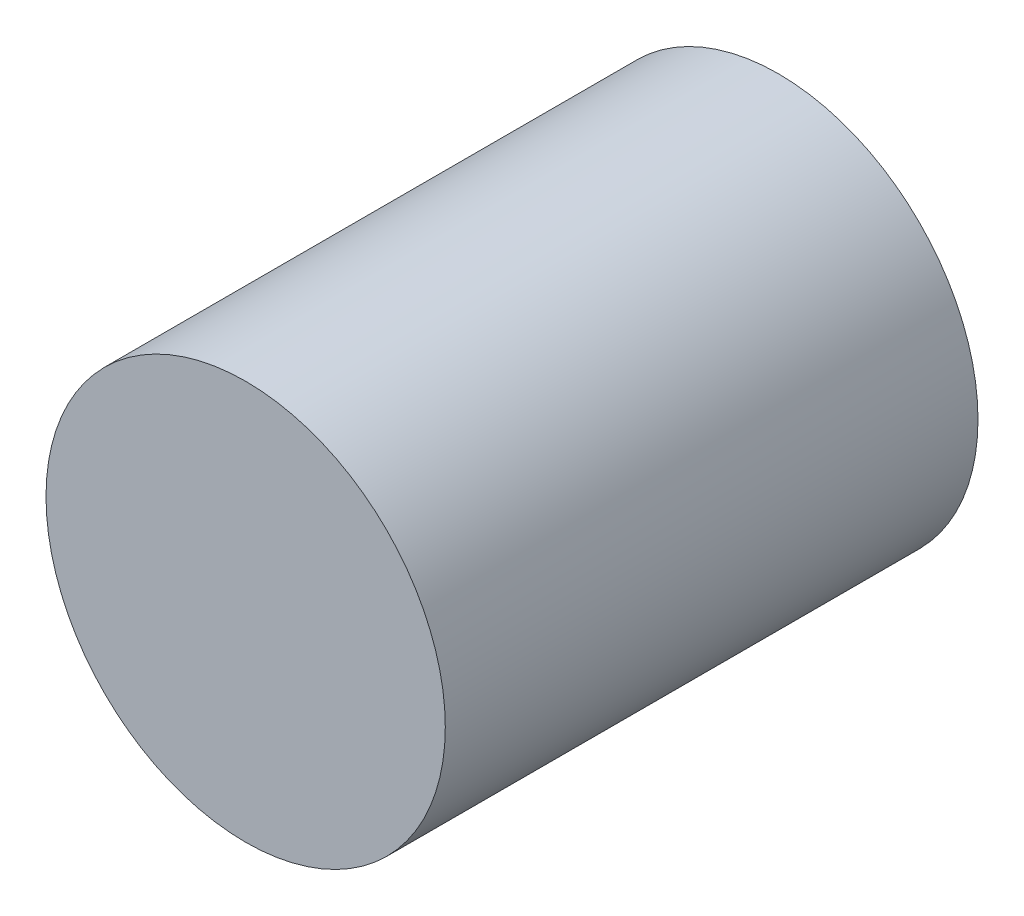
SolidWorks part; units mm, degrees
material "Plain Carbon Steel"
ref_plane "Front Plane" through (0, 0, 0) normal (0, 0, 1) x (1, 0, 0)
ref_plane "Top Plane" through (0, 0, 0) normal (0, 1, 0) x (1, 0, 0)
ref_plane "Right Plane" through (0, 0, 0) normal (1, 0, 0) x (0, 0, -1)
sketch "Pin Profile Ø9.52" plane through (0, 0, 0) normal (0, 0, 1) x (1, 0, 0)
  circle A0 centre (0, 0) radius 4.76
  dimension "D1" = 9.52
extrude "Pin Body Extrude 12.7" add sketch "Pin Profile Ø9.52" along normal blind 12.7
